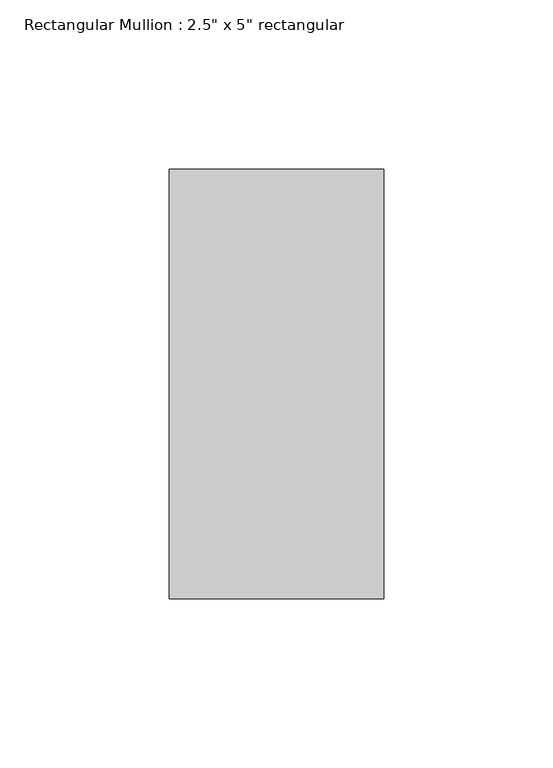
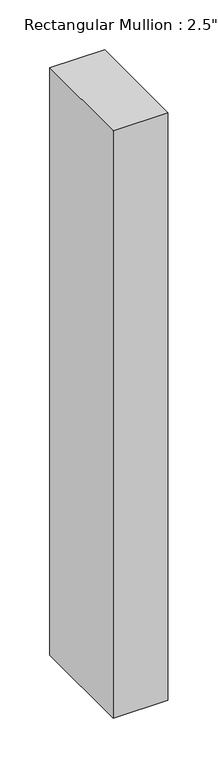
"""IFC4 building model written with IfcOpenShell, lengths in millimetres: member geometry."""

from ifc_helpers import new_model, si_unit, frame, origin, place, context, project, spatial, polyline, outline, extrude, source, transform, mapped, element, save


def member_a86422a6(model_context):
    return source(origin(), model_context, "Body", "SweptSolid", [
        extrude(outline(polyline([(31.75, 63.5), (31.75, -63.5), (-31.75, -63.5), (-31.75, 63.5), (31.75, 63.5)])), frame((0.0, 0.0, -719.6039078), z_axis=(0.0, 0.0, 1.0), x_axis=(1.0, 0.0, 0.0)), (0.0, 0.0, 1.0), 719.6039078),
    ])


if __name__ == "__main__":
    model = new_model("IFC4")
    model_context = context("Model", 3, world=origin())
    ifc_project = project(units=[si_unit("LENGTHUNIT", "METRE", prefix="MILLI")], contexts=[model_context])
    site = spatial("IfcSite", under=ifc_project)
    building = spatial("IfcBuilding", under=site)
    placement = place(None, origin())
    member_shape = member_a86422a6(model_context)
    element("IfcMember", 1, ObjectType="Rectangular Mullion : 2.5\" x 5\" rectangular", at=placement, inside=building, context=model_context, shape_type="MappedRepresentation", body=[
        mapped(member_shape, transform((0.0, 0.0, 0.0), x_axis=(1.0, 0.0, 0.0), y_axis=(0.0, 1.0, 0.0), z_axis=(0.0, 0.0, 1.0))),
    ])
    save(model, "model.ifc")

# Revit data of these elements
# Type "Rectangular Mullion : 2.5\" x 5\" rectangular"
#   built-in parameter 1007304 = 0.416667 (stored number, unit not read)
#   built-in parameter 1007301 = 0.104167 (stored number, unit not read)
#   built-in parameter 1007300 = 0.104167 (stored number, unit not read)
# Element 1 (IfcMember, "Rectangular Mullion : 2.5\" x 5\" rectangular")
#   Materials on its faces: "Aluminum"
# Materials
#   "Aluminum": class "Metal", colour RGB 247 247 247, transparency 0, Description = "Aluminum 6061", Cost = 0
